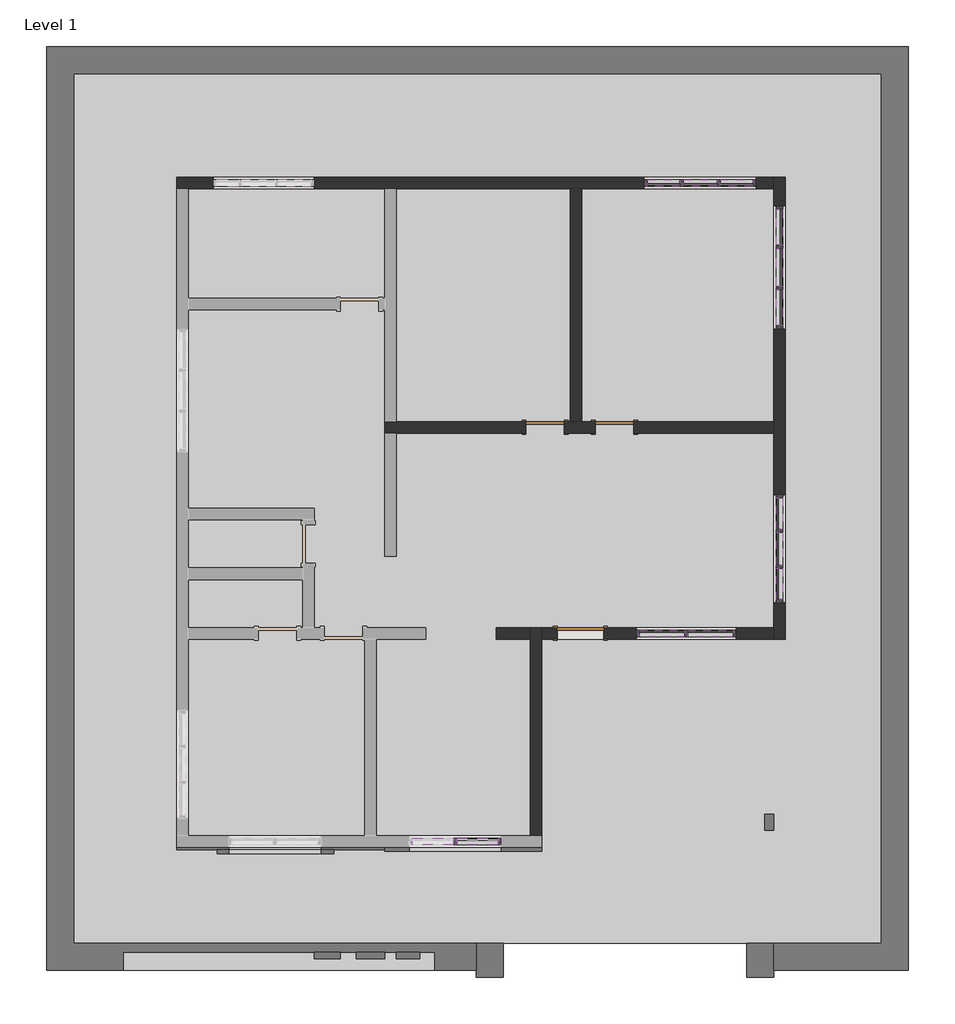
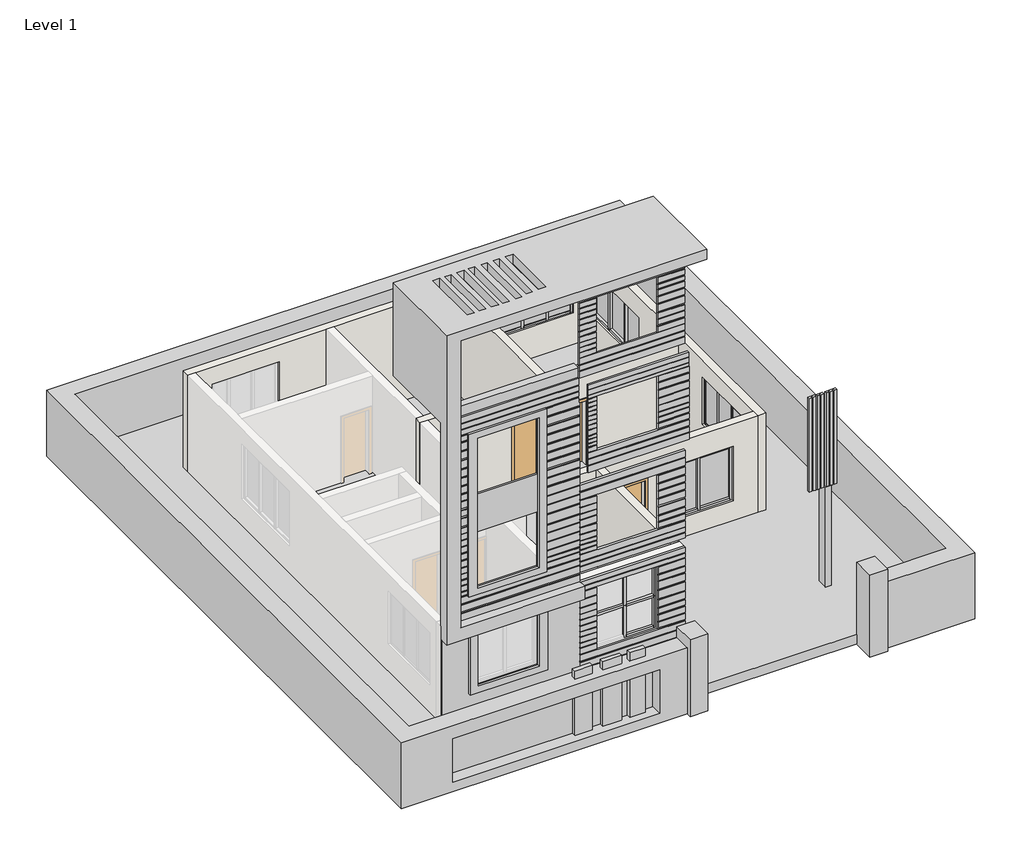
# One storey, part 2 of 2: 46 members, 11 plates, 7 walls, 3 doors, 3 proxies.
"""IFC4 building model written with IfcOpenShell, lengths in millimetres."""

from ifc_helpers import new_model, si_unit, frame, origin, origin_with_axes, place, context, project, spatial, polyline, outline, extrude, faceted_brep, transform, mapped, element, save
from components import generic_models_1_generic_models_1_92ce0f77, generic_models_7_generic_models_7_680a3b92, generic_models_7_generic_models_7_94141b15, generic_models_8_generic_models_8_408287a0, door_a1484949, door_85036156, door_a90ba1ad, member_3f0e0172, member_5215b92c, member_673fd8de, member_e79a7e0a, member_9d02be77, member_7007ad49, member_d44a35f4, member_12fb2005, member_61359a5b, member_26d576e8, member_7f309565, member_d4c304d5, member_f1f71bde, member_07726a47, member_145ad7ec, member_948b814d, member_c17f1be2, member_ad567e07, member_e156fde9, system_panel_glazed_296d4335, system_panel_glazed_a5c0bc7c, system_panel_glazed_82717b58, system_panel_glazed_5516fd1f, system_panel_glazed_95f8db0f, system_panel_glazed_7e52d88a, system_panel_glazed_d1fbebc5

model = new_model("IFC4")

# Units and contexts
model_context = context("Model", 3, world=origin())
ifc_project = project(units=[si_unit("LENGTHUNIT", "METRE", prefix="MILLI")], contexts=[model_context])

# Site, building, storey
site = spatial("IfcSite", under=ifc_project)
building = spatial("IfcBuilding", under=site)
storey = spatial("IfcBuildingStorey", under=building, Name="Level 1", Elevation=0.0)

# Proxies
placement = place(None, origin())
generic_models_1_generic_models_1_shape = generic_models_1_generic_models_1_92ce0f77(model_context)
element("IfcBuildingElementProxy", 1, Name="Generic Models 1 : Generic Models 1", ObjectType="Generic Models 1 : Generic Models 1", at=placement, inside=storey, context=model_context, shape_type="MappedRepresentation", body=[
    mapped(generic_models_1_generic_models_1_shape, transform((0.0, 0.0, 0.0), x_axis=(1.0, 0.0, 0.0), y_axis=(0.0, 1.0, 0.0), z_axis=(0.0, 0.0, 1.0))),
])
generic_models_7_generic_models_7_shape = generic_models_7_generic_models_7_680a3b92(model_context)
generic_models_7_generic_models_7_2_shape = generic_models_7_generic_models_7_94141b15(model_context)
element("IfcBuildingElementProxy", 2, Name="Generic Models 7 : Generic Models 7", ObjectType="Generic Models 7 : Generic Models 7", at=placement, inside=storey, context=model_context, shape_type="MappedRepresentation", body=[
    mapped(generic_models_7_generic_models_7_shape, transform((0.0, 0.0, 0.0), x_axis=(1.0, 0.0, 0.0), y_axis=(0.0, 1.0, 0.0), z_axis=(0.0, 0.0, 1.0))),
    mapped(generic_models_7_generic_models_7_2_shape, transform((0.0, 0.0, 0.0), x_axis=(1.0, 0.0, 0.0), y_axis=(0.0, 1.0, 0.0), z_axis=(0.0, 0.0, 1.0))),
])
generic_models_8_generic_models_8_shape = generic_models_8_generic_models_8_408287a0(model_context)
element("IfcBuildingElementProxy", 3, Name="Generic Models 8 : Generic Models 8", ObjectType="Generic Models 8 : Generic Models 8", at=placement, inside=storey, context=model_context, shape_type="MappedRepresentation", body=[
    mapped(generic_models_8_generic_models_8_shape, transform((0.0, 0.0, 0.0), x_axis=(1.0, 0.0, 0.0), y_axis=(0.0, 1.0, 0.0), z_axis=(0.0, 0.0, 1.0))),
])

# Doors
door_shape = door_a1484949(model_context)
element("IfcDoor", 4, ObjectType="Single-Flush : 30\" x 80\"", at=placement, inside=storey, context=model_context, shape_type="MappedRepresentation", body=[
    mapped(door_shape, transform((-12995.791855, -5548.3538163, 0.0), x_axis=(1.0, 0.0, 0.0), y_axis=(0.0, 1.0, 0.0), z_axis=(0.0, 0.0, 1.0))),
])
door_2_shape = door_85036156(model_context)
element("IfcDoor", 5, ObjectType="Single-Flush : 30\" x 80\"", at=placement, inside=storey, context=model_context, shape_type="MappedRepresentation", body=[
    mapped(door_2_shape, transform((-11624.191855, -5548.3538163, 0.0), x_axis=(-1.0, 0.0, 0.0), y_axis=(0.0, -1.0, 0.0), z_axis=(0.0, 0.0, 1.0))),
])
door_3_shape = door_a90ba1ad(model_context)
element("IfcDoor", 6, ObjectType="Single-Flush : 36\" x 84\"", at=placement, inside=storey, context=model_context, shape_type="MappedRepresentation", body=[
    mapped(door_3_shape, transform((-12297.291855, -9625.0538163, 50.8), x_axis=(-1.0, 0.0, 0.0), y_axis=(0.0, -1.0, 0.0), z_axis=(0.0, 0.0, 1.0))),
])

# Members
member_shape = member_3f0e0172(model_context)
element("IfcMember", 7, ObjectType="Rectangular Mullion : 2.5\" x 5\" rectangular", at=placement, inside=storey, context=model_context, shape_type="MappedRepresentation", body=[
    mapped(member_shape, transform((-8360.291855, -7561.3038163, 1043.4119261), x_axis=(0.0, 0.0, -1.0), y_axis=(1.0, 0.0, 0.0), z_axis=(0.0, -1.0, 0.0))),
])
element("IfcMember", 8, ObjectType="Rectangular Mullion : 2.5\" x 5\" rectangular", at=placement, inside=storey, context=model_context, shape_type="MappedRepresentation", body=[
    mapped(member_shape, transform((-8360.291855, -8951.9538163, 1043.4119261), x_axis=(0.0, 0.0, -1.0), y_axis=(1.0, 0.0, 0.0), z_axis=(0.0, -1.0, 0.0))),
])
member_2_shape = member_5215b92c(model_context)
element("IfcMember", 9, ObjectType="Rectangular Mullion : 2.5\" x 5\" rectangular", at=placement, inside=storey, context=model_context, shape_type="MappedRepresentation", body=[
    mapped(member_2_shape, transform((-8360.291855, -8272.5038163, 1043.4119261), x_axis=(0.0, 0.0, -1.0), y_axis=(1.0, 0.0, 0.0), z_axis=(0.0, -1.0, 0.0))),
])
member_3_shape = member_673fd8de(model_context)
element("IfcMember", 10, ObjectType="Rectangular Mullion : 2.5\" x 5\" rectangular", at=placement, inside=storey, context=model_context, shape_type="MappedRepresentation", body=[
    mapped(member_3_shape, transform((-8360.291855, -8304.2538163, 1043.4119261), x_axis=(0.0, 1.0, 0.0), y_axis=(1.0, 0.0, 0.0), z_axis=(0.0, 0.0, -1.0))),
])
element("IfcMember", 11, ObjectType="Rectangular Mullion : 2.5\" x 5\" rectangular", at=placement, inside=storey, context=model_context, shape_type="MappedRepresentation", body=[
    mapped(member_3_shape, transform((-8360.291855, -7593.0538163, 1043.4119261), x_axis=(0.0, 1.0, 0.0), y_axis=(1.0, 0.0, 0.0), z_axis=(0.0, 0.0, -1.0))),
])
element("IfcMember", 12, ObjectType="Rectangular Mullion : 2.5\" x 5\" rectangular", at=placement, inside=storey, context=model_context, shape_type="MappedRepresentation", body=[
    mapped(member_2_shape, transform((-8360.291855, -7624.8038163, 2519.2132879), x_axis=(0.0, 0.0, 1.0), y_axis=(1.0, 0.0, 0.0), z_axis=(0.0, 1.0, 0.0))),
])
element("IfcMember", 13, ObjectType="Rectangular Mullion : 2.5\" x 5\" rectangular", at=placement, inside=storey, context=model_context, shape_type="MappedRepresentation", body=[
    mapped(member_shape, transform((-8360.291855, -8336.0038163, 2519.2132879), x_axis=(0.0, 0.0, 1.0), y_axis=(1.0, 0.0, 0.0), z_axis=(0.0, 1.0, 0.0))),
])
element("IfcMember", 14, ObjectType="Rectangular Mullion : 2.5\" x 5\" rectangular", at=placement, inside=storey, context=model_context, shape_type="MappedRepresentation", body=[
    mapped(member_shape, transform((-8360.291855, -6945.3538163, 2519.2132879), x_axis=(0.0, 0.0, 1.0), y_axis=(1.0, 0.0, 0.0), z_axis=(0.0, 1.0, 0.0))),
])
member_4_shape = member_e79a7e0a(model_context)
element("IfcMember", 15, ObjectType="Rectangular Mullion : 2.5\" x 5\" rectangular", at=placement, inside=storey, context=model_context, shape_type="MappedRepresentation", body=[
    mapped(member_4_shape, transform((-8360.291855, -6881.8538163, 1043.4119261), x_axis=(0.0, 1.0, 0.0), y_axis=(1.0, 0.0, 0.0), z_axis=(0.0, 0.0, -1.0))),
])
element("IfcMember", 16, ObjectType="Rectangular Mullion : 2.5\" x 5\" rectangular", at=placement, inside=storey, context=model_context, shape_type="MappedRepresentation", body=[
    mapped(member_4_shape, transform((-8360.291855, -9015.4538163, 2519.2132879), x_axis=(0.0, -1.0, 0.0), y_axis=(1.0, 0.0, 0.0), z_axis=(0.0, 0.0, 1.0))),
])
member_5_shape = member_9d02be77(model_context)
element("IfcMember", 17, ObjectType="Rectangular Mullion : 2.5\" x 5\" rectangular", at=placement, inside=storey, context=model_context, shape_type="MappedRepresentation", body=[
    mapped(member_5_shape, transform((-8360.291855, -2011.4038163, 996.5765581), x_axis=(0.0, 0.0, -1.0), y_axis=(-1.0, 0.0, 0.0), z_axis=(0.0, 1.0, 0.0))),
])
member_6_shape = member_7007ad49(model_context)
element("IfcMember", 18, ObjectType="Rectangular Mullion : 2.5\" x 5\" rectangular", at=placement, inside=storey, context=model_context, shape_type="MappedRepresentation", body=[
    mapped(member_6_shape, transform((-8360.291855, -2824.2038163, 996.5765581), x_axis=(0.0, 0.0, -1.0), y_axis=(-1.0, 0.0, 0.0), z_axis=(0.0, 1.0, 0.0))),
])
element("IfcMember", 19, ObjectType="Rectangular Mullion : 2.5\" x 5\" rectangular", at=placement, inside=storey, context=model_context, shape_type="MappedRepresentation", body=[
    mapped(member_6_shape, transform((-8360.291855, -1230.3538163, 996.5765581), x_axis=(0.0, 0.0, -1.0), y_axis=(-1.0, 0.0, 0.0), z_axis=(0.0, 1.0, 0.0))),
])
member_7_shape = member_d44a35f4(model_context)
element("IfcMember", 20, ObjectType="Rectangular Mullion : 2.5\" x 5\" rectangular", at=placement, inside=storey, context=model_context, shape_type="MappedRepresentation", body=[
    mapped(member_7_shape, transform((-8360.291855, -1979.6538163, 996.5765581), x_axis=(0.0, -1.0, 0.0), y_axis=(-1.0, 0.0, 0.0), z_axis=(0.0, 0.0, -1.0))),
])
element("IfcMember", 21, ObjectType="Rectangular Mullion : 2.5\" x 5\" rectangular", at=placement, inside=storey, context=model_context, shape_type="MappedRepresentation", body=[
    mapped(member_7_shape, transform((-8360.291855, -2792.4538163, 996.5765581), x_axis=(0.0, -1.0, 0.0), y_axis=(-1.0, 0.0, 0.0), z_axis=(0.0, 0.0, -1.0))),
])
element("IfcMember", 22, ObjectType="Rectangular Mullion : 2.5\" x 5\" rectangular", at=placement, inside=storey, context=model_context, shape_type="MappedRepresentation", body=[
    mapped(member_6_shape, transform((-8360.291855, -1947.9038163, 2408.3673873), x_axis=(0.0, 0.0, 1.0), y_axis=(-1.0, 0.0, 0.0), z_axis=(0.0, -1.0, 0.0))),
])
element("IfcMember", 23, ObjectType="Rectangular Mullion : 2.5\" x 5\" rectangular", at=placement, inside=storey, context=model_context, shape_type="MappedRepresentation", body=[
    mapped(member_6_shape, transform((-8360.291855, -3541.7538163, 2408.3673873), x_axis=(0.0, 0.0, 1.0), y_axis=(-1.0, 0.0, 0.0), z_axis=(0.0, -1.0, 0.0))),
])
element("IfcMember", 24, ObjectType="Rectangular Mullion : 2.5\" x 5\" rectangular", at=placement, inside=storey, context=model_context, shape_type="MappedRepresentation", body=[
    mapped(member_5_shape, transform((-8360.291855, -2760.7038163, 2408.3673873), x_axis=(0.0, 0.0, 1.0), y_axis=(-1.0, 0.0, 0.0), z_axis=(0.0, -1.0, 0.0))),
])
member_8_shape = member_12fb2005(model_context)
element("IfcMember", 25, ObjectType="Rectangular Mullion : 2.5\" x 5\" rectangular", at=placement, inside=storey, context=model_context, shape_type="MappedRepresentation", body=[
    mapped(member_8_shape, transform((-8360.291855, -3605.2538163, 996.5765581), x_axis=(0.0, -1.0, 0.0), y_axis=(-1.0, 0.0, 0.0), z_axis=(0.0, 0.0, -1.0))),
])
element("IfcMember", 26, ObjectType="Rectangular Mullion : 2.5\" x 5\" rectangular", at=placement, inside=storey, context=model_context, shape_type="MappedRepresentation", body=[
    mapped(member_8_shape, transform((-8360.291855, -1166.8538163, 2408.3673873), x_axis=(0.0, 1.0, 0.0), y_axis=(-1.0, 0.0, 0.0), z_axis=(0.0, 0.0, 1.0))),
])
member_9_shape = member_61359a5b(model_context)
element("IfcMember", 27, ObjectType="Rectangular Mullion : 2.5\" x 5\" rectangular", at=placement, inside=storey, context=model_context, shape_type="MappedRepresentation", body=[
    mapped(member_9_shape, transform((-9526.5751883, -709.6538163, 2499.4975793), x_axis=(0.0, 0.0, 1.0), y_axis=(0.0, 1.0, 0.0), z_axis=(-1.0, 0.0, 0.0))),
])
element("IfcMember", 28, ObjectType="Rectangular Mullion : 2.5\" x 5\" rectangular", at=placement, inside=storey, context=model_context, shape_type="MappedRepresentation", body=[
    mapped(member_9_shape, transform((-10976.491855, -709.6538163, 2499.4975793), x_axis=(0.0, 0.0, 1.0), y_axis=(0.0, 1.0, 0.0), z_axis=(-1.0, 0.0, 0.0))),
])
member_10_shape = member_26d576e8(model_context)
element("IfcMember", 29, ObjectType="Rectangular Mullion : 2.5\" x 5\" rectangular", at=placement, inside=storey, context=model_context, shape_type="MappedRepresentation", body=[
    mapped(member_10_shape, transform((-10267.4085217, -709.6538163, 2499.4975793), x_axis=(0.0, 0.0, 1.0), y_axis=(0.0, 1.0, 0.0), z_axis=(-1.0, 0.0, 0.0))),
])
member_11_shape = member_7f309565(model_context)
element("IfcMember", 30, ObjectType="Rectangular Mullion : 2.5\" x 5\" rectangular", at=placement, inside=storey, context=model_context, shape_type="MappedRepresentation", body=[
    mapped(member_11_shape, transform((-10299.1585217, -709.6538163, 985.9213876), x_axis=(-1.0, 0.0, 0.0), y_axis=(0.0, 1.0, 0.0), z_axis=(0.0, 0.0, -1.0))),
])
element("IfcMember", 31, ObjectType="Rectangular Mullion : 2.5\" x 5\" rectangular", at=placement, inside=storey, context=model_context, shape_type="MappedRepresentation", body=[
    mapped(member_11_shape, transform((-9558.3251883, -709.6538163, 985.9213876), x_axis=(-1.0, 0.0, 0.0), y_axis=(0.0, 1.0, 0.0), z_axis=(0.0, 0.0, -1.0))),
])
element("IfcMember", 32, ObjectType="Rectangular Mullion : 2.5\" x 5\" rectangular", at=placement, inside=storey, context=model_context, shape_type="MappedRepresentation", body=[
    mapped(member_10_shape, transform((-9590.0751883, -709.6538163, 985.9213876), x_axis=(0.0, 0.0, -1.0), y_axis=(0.0, 1.0, 0.0), z_axis=(1.0, 0.0, 0.0))),
])
element("IfcMember", 33, ObjectType="Rectangular Mullion : 2.5\" x 5\" rectangular", at=placement, inside=storey, context=model_context, shape_type="MappedRepresentation", body=[
    mapped(member_9_shape, transform((-10330.9085217, -709.6538163, 985.9213876), x_axis=(0.0, 0.0, -1.0), y_axis=(0.0, 1.0, 0.0), z_axis=(1.0, 0.0, 0.0))),
])
element("IfcMember", 34, ObjectType="Rectangular Mullion : 2.5\" x 5\" rectangular", at=placement, inside=storey, context=model_context, shape_type="MappedRepresentation", body=[
    mapped(member_9_shape, transform((-8880.991855, -709.6538163, 985.9213876), x_axis=(0.0, 0.0, -1.0), y_axis=(0.0, 1.0, 0.0), z_axis=(1.0, 0.0, 0.0))),
])
member_12_shape = member_d4c304d5(model_context)
element("IfcMember", 35, ObjectType="Rectangular Mullion : 2.5\" x 5\" rectangular", at=placement, inside=storey, context=model_context, shape_type="MappedRepresentation", body=[
    mapped(member_12_shape, transform((-11039.991855, -709.6538163, 985.9213876), x_axis=(-1.0, 0.0, 0.0), y_axis=(0.0, 1.0, 0.0), z_axis=(0.0, 0.0, -1.0))),
])
element("IfcMember", 36, ObjectType="Rectangular Mullion : 2.5\" x 5\" rectangular", at=placement, inside=storey, context=model_context, shape_type="MappedRepresentation", body=[
    mapped(member_12_shape, transform((-8817.491855, -709.6538163, 2499.4975793), x_axis=(1.0, 0.0, 0.0), y_axis=(0.0, 1.0, 0.0), z_axis=(0.0, 0.0, 1.0))),
])
member_13_shape = member_f1f71bde(model_context)
element("IfcMember", 37, ObjectType="Rectangular Mullion : 2.5\" x 5\" rectangular", at=placement, inside=storey, context=model_context, shape_type="MappedRepresentation", body=[
    mapped(member_13_shape, transform((-10233.541855, -9625.0538163, 2332.3247485), x_axis=(0.0, 0.0, 1.0), y_axis=(0.0, -1.0, 0.0), z_axis=(1.0, 0.0, 0.0))),
])
element("IfcMember", 38, ObjectType="Rectangular Mullion : 2.5\" x 5\" rectangular", at=placement, inside=storey, context=model_context, shape_type="MappedRepresentation", body=[
    mapped(member_13_shape, transform((-9274.691855, -9625.0538163, 2332.3247485), x_axis=(0.0, 0.0, 1.0), y_axis=(0.0, -1.0, 0.0), z_axis=(1.0, 0.0, 0.0))),
])
member_14_shape = member_07726a47(model_context)
element("IfcMember", 39, ObjectType="Rectangular Mullion : 2.5\" x 5\" rectangular", at=placement, inside=storey, context=model_context, shape_type="MappedRepresentation", body=[
    mapped(member_14_shape, transform((-10201.791855, -9625.0538163, 631.9229902), x_axis=(1.0, 0.0, 0.0), y_axis=(0.0, -1.0, 0.0), z_axis=(0.0, 0.0, -1.0))),
])
element("IfcMember", 40, ObjectType="Rectangular Mullion : 2.5\" x 5\" rectangular", at=placement, inside=storey, context=model_context, shape_type="MappedRepresentation", body=[
    mapped(member_13_shape, transform((-10170.041855, -9625.0538163, 631.9229902), x_axis=(0.0, 0.0, -1.0), y_axis=(0.0, -1.0, 0.0), z_axis=(-1.0, 0.0, 0.0))),
])
element("IfcMember", 41, ObjectType="Rectangular Mullion : 2.5\" x 5\" rectangular", at=placement, inside=storey, context=model_context, shape_type="MappedRepresentation", body=[
    mapped(member_13_shape, transform((-11128.891855, -9625.0538163, 631.9229902), x_axis=(0.0, 0.0, -1.0), y_axis=(0.0, -1.0, 0.0), z_axis=(-1.0, 0.0, 0.0))),
])
member_15_shape = member_145ad7ec(model_context)
element("IfcMember", 42, ObjectType="Rectangular Mullion : 2.5\" x 5\" rectangular", at=placement, inside=storey, context=model_context, shape_type="MappedRepresentation", body=[
    mapped(member_15_shape, transform((-9211.191855, -9625.0538163, 631.9229902), x_axis=(1.0, 0.0, 0.0), y_axis=(0.0, -1.0, 0.0), z_axis=(0.0, 0.0, -1.0))),
])
element("IfcMember", 43, ObjectType="Rectangular Mullion : 2.5\" x 5\" rectangular", at=placement, inside=storey, context=model_context, shape_type="MappedRepresentation", body=[
    mapped(member_15_shape, transform((-11192.391855, -9625.0538163, 2332.3247485), x_axis=(-1.0, 0.0, 0.0), y_axis=(0.0, -1.0, 0.0), z_axis=(0.0, 0.0, 1.0))),
])
member_16_shape = member_948b814d(model_context)
element("IfcMember", 44, ObjectType="Rectangular Mullion : 2.5\" x 5\" rectangular", at=placement, inside=storey, context=model_context, shape_type="MappedRepresentation", body=[
    mapped(member_16_shape, transform((-14773.791855, -13739.8538163, 1742.3683755), x_axis=(1.0, 0.0, 0.0), y_axis=(0.0, -1.0, 0.0), z_axis=(0.0, 0.0, -1.0))),
])
member_17_shape = member_c17f1be2(model_context)
element("IfcMember", 45, ObjectType="Rectangular Mullion : 2.5\" x 5\" rectangular", at=placement, inside=storey, context=model_context, shape_type="MappedRepresentation", body=[
    mapped(member_17_shape, transform((-14805.541855, -13739.8538163, 2743.3706019), x_axis=(0.0, 0.0, 1.0), y_axis=(0.0, -1.0, 0.0), z_axis=(1.0, 0.0, 0.0))),
])
element("IfcMember", 46, ObjectType="Rectangular Mullion : 2.5\" x 5\" rectangular", at=placement, inside=storey, context=model_context, shape_type="MappedRepresentation", body=[
    mapped(member_17_shape, transform((-13922.891855, -13739.8538163, 2743.3706019), x_axis=(0.0, 0.0, 1.0), y_axis=(0.0, -1.0, 0.0), z_axis=(1.0, 0.0, 0.0))),
])
member_18_shape = member_ad567e07(model_context)
element("IfcMember", 47, ObjectType="Rectangular Mullion : 2.5\" x 5\" rectangular", at=placement, inside=storey, context=model_context, shape_type="MappedRepresentation", body=[
    mapped(member_18_shape, transform((-13922.891855, -13739.8538163, 1742.3683755), x_axis=(0.0, 0.0, 1.0), y_axis=(0.0, -1.0, 0.0), z_axis=(1.0, 0.0, 0.0))),
])
element("IfcMember", 48, ObjectType="Rectangular Mullion : 2.5\" x 5\" rectangular", at=placement, inside=storey, context=model_context, shape_type="MappedRepresentation", body=[
    mapped(member_18_shape, transform((-14805.541855, -13739.8538163, 1742.3683755), x_axis=(0.0, 0.0, 1.0), y_axis=(0.0, -1.0, 0.0), z_axis=(1.0, 0.0, 0.0))),
])
member_19_shape = member_e156fde9(model_context)
element("IfcMember", 49, ObjectType="Rectangular Mullion : 2.5\" x 5\" rectangular", at=placement, inside=storey, context=model_context, shape_type="MappedRepresentation", body=[
    mapped(member_19_shape, transform((-13859.391855, -13739.8538163, 1742.3683755), x_axis=(1.0, 0.0, 0.0), y_axis=(0.0, -1.0, 0.0), z_axis=(0.0, 0.0, -1.0))),
])
element("IfcMember", 50, ObjectType="Rectangular Mullion : 2.5\" x 5\" rectangular", at=placement, inside=storey, context=model_context, shape_type="MappedRepresentation", body=[
    mapped(member_16_shape, transform((-14773.791855, -13739.8538163, 741.3661492), x_axis=(1.0, 0.0, 0.0), y_axis=(0.0, -1.0, 0.0), z_axis=(0.0, 0.0, -1.0))),
])
element("IfcMember", 51, ObjectType="Rectangular Mullion : 2.5\" x 5\" rectangular", at=placement, inside=storey, context=model_context, shape_type="MappedRepresentation", body=[
    mapped(member_17_shape, transform((-14742.041855, -13739.8538163, 741.3661492), x_axis=(0.0, 0.0, -1.0), y_axis=(0.0, -1.0, 0.0), z_axis=(-1.0, 0.0, 0.0))),
])
element("IfcMember", 52, ObjectType="Rectangular Mullion : 2.5\" x 5\" rectangular", at=placement, inside=storey, context=model_context, shape_type="MappedRepresentation", body=[
    mapped(member_19_shape, transform((-13859.391855, -13739.8538163, 741.3661492), x_axis=(1.0, 0.0, 0.0), y_axis=(0.0, -1.0, 0.0), z_axis=(0.0, 0.0, -1.0))),
])

# Plates
system_panel_glazed_shape = system_panel_glazed_296d4335(model_context)
element("IfcPlate", 53, ObjectType="System Panel : Glazed", at=placement, inside=storey, context=model_context, shape_type="MappedRepresentation", body=[
    mapped(system_panel_glazed_shape, transform((-8360.291855, -8643.9788163, 1106.9119261), x_axis=(0.0, 1.0, 0.0), y_axis=(-1.0, 0.0, 0.0), z_axis=(0.0, 0.0, 1.0))),
])
element("IfcPlate", 54, ObjectType="System Panel : Glazed", at=placement, inside=storey, context=model_context, shape_type="MappedRepresentation", body=[
    mapped(system_panel_glazed_shape, transform((-8360.291855, -7253.3288163, 1106.9119261), x_axis=(0.0, 1.0, 0.0), y_axis=(-1.0, 0.0, 0.0), z_axis=(0.0, 0.0, 1.0))),
])
system_panel_glazed_2_shape = system_panel_glazed_a5c0bc7c(model_context)
element("IfcPlate", 55, ObjectType="System Panel : Glazed", at=placement, inside=storey, context=model_context, shape_type="MappedRepresentation", body=[
    mapped(system_panel_glazed_2_shape, transform((-8360.291855, -7948.6538163, 1106.9119261), x_axis=(0.0, 1.0, 0.0), y_axis=(-1.0, 0.0, 0.0), z_axis=(0.0, 0.0, 1.0))),
])
system_panel_glazed_3_shape = system_panel_glazed_82717b58(model_context)
element("IfcPlate", 56, ObjectType="System Panel : Glazed", at=placement, inside=storey, context=model_context, shape_type="MappedRepresentation", body=[
    mapped(system_panel_glazed_3_shape, transform((-8360.291855, -1589.1288163, 1060.0765581), x_axis=(0.0, -1.0, 0.0), y_axis=(1.0, 0.0, 0.0), z_axis=(0.0, 0.0, 1.0))),
])
element("IfcPlate", 57, ObjectType="System Panel : Glazed", at=placement, inside=storey, context=model_context, shape_type="MappedRepresentation", body=[
    mapped(system_panel_glazed_3_shape, transform((-8360.291855, -3182.9788163, 1060.0765581), x_axis=(0.0, -1.0, 0.0), y_axis=(1.0, 0.0, 0.0), z_axis=(0.0, 0.0, 1.0))),
])
system_panel_glazed_4_shape = system_panel_glazed_5516fd1f(model_context)
element("IfcPlate", 58, ObjectType="System Panel : Glazed", at=placement, inside=storey, context=model_context, shape_type="MappedRepresentation", body=[
    mapped(system_panel_glazed_4_shape, transform((-8360.291855, -2386.0538163, 1060.0765581), x_axis=(0.0, -1.0, 0.0), y_axis=(1.0, 0.0, 0.0), z_axis=(0.0, 0.0, 1.0))),
])
system_panel_glazed_5_shape = system_panel_glazed_95f8db0f(model_context)
element("IfcPlate", 59, ObjectType="System Panel : Glazed", at=placement, inside=storey, context=model_context, shape_type="MappedRepresentation", body=[
    mapped(system_panel_glazed_5_shape, transform((-9203.7835217, -709.6538163, 1049.4213876), x_axis=(-1.0, 0.0, 0.0), y_axis=(0.0, -1.0, 0.0), z_axis=(0.0, 0.0, 1.0))),
])
element("IfcPlate", 60, ObjectType="System Panel : Glazed", at=placement, inside=storey, context=model_context, shape_type="MappedRepresentation", body=[
    mapped(system_panel_glazed_5_shape, transform((-10653.7001883, -709.6538163, 1049.4213876), x_axis=(-1.0, 0.0, 0.0), y_axis=(0.0, -1.0, 0.0), z_axis=(0.0, 0.0, 1.0))),
])
system_panel_glazed_6_shape = system_panel_glazed_7e52d88a(model_context)
element("IfcPlate", 61, ObjectType="System Panel : Glazed", at=placement, inside=storey, context=model_context, shape_type="MappedRepresentation", body=[
    mapped(system_panel_glazed_6_shape, transform((-9928.741855, -709.6538163, 1049.4213876), x_axis=(-1.0, 0.0, 0.0), y_axis=(0.0, -1.0, 0.0), z_axis=(0.0, 0.0, 1.0))),
])
system_panel_glazed_7_shape = system_panel_glazed_d1fbebc5(model_context)
element("IfcPlate", 62, ObjectType="System Panel : Glazed", at=placement, inside=storey, context=model_context, shape_type="MappedRepresentation", body=[
    mapped(system_panel_glazed_7_shape, transform((-10681.216855, -9625.0538163, 695.4229902), x_axis=(1.0, 0.0, 0.0), y_axis=(0.0, 1.0, 0.0), z_axis=(0.0, 0.0, 1.0))),
])
element("IfcPlate", 63, ObjectType="System Panel : Glazed", at=placement, inside=storey, context=model_context, shape_type="MappedRepresentation", body=[
    mapped(system_panel_glazed_7_shape, transform((-9722.366855, -9625.0538163, 695.4229902), x_axis=(1.0, 0.0, 0.0), y_axis=(0.0, 1.0, 0.0), z_axis=(0.0, 0.0, 1.0))),
])

# Walls
element("IfcWall", 64, ObjectType="9\"", at=placement, inside=storey, context=model_context, shape_type="Brep", body=[
    faceted_brep([(-8474.591855, -595.3538163, 0.0), (-20285.591855, -595.3538163, 0.0), (-20285.591855, -595.3538163, 3048.0), (-8474.591855, -595.3538163, 3048.0), (-8817.491855, -595.3538163, 985.9213876), (-8817.491855, -595.3538163, 2499.4975793), (-11039.991855, -595.3538163, 2499.4975793), (-11039.991855, -595.3538163, 985.9213876), (-19561.691855, -595.3538163, 2512.1183195), (-19561.691855, -595.3538163, 954.7607085), (-17567.791855, -595.3538163, 954.7607085), (-17567.791855, -595.3538163, 2512.1183195), (-20285.591855, -823.9538163, 0.0), (-20056.991855, -823.9538163, 0.0), (-16170.791855, -823.9538163, 0.0), (-15942.191855, -823.9538163, 0.0), (-12500.491855, -823.9538163, 0.0), (-12271.891855, -823.9538163, 0.0), (-8474.591855, -823.9538163, 0.0), (-8474.591855, -823.9538163, 3048.0), (-12271.891855, -823.9538163, 3048.0), (-12500.491855, -823.9538163, 3048.0), (-15942.191855, -823.9538163, 3048.0), (-16170.791855, -823.9538163, 3048.0), (-20056.991855, -823.9538163, 3048.0), (-20285.591855, -823.9538163, 3048.0), (-8817.491855, -823.9538163, 2499.4975793), (-8817.491855, -823.9538163, 985.9213876), (-11039.991855, -823.9538163, 985.9213876), (-11039.991855, -823.9538163, 2499.4975793), (-19561.691855, -823.9538163, 954.7607085), (-19561.691855, -823.9538163, 2512.1183195), (-17567.791855, -823.9538163, 2512.1183195), (-17567.791855, -823.9538163, 954.7607085)], [[[0, 1, 2, 3], [4, 5, 6, 7], [8, 9, 10, 11]], [[12, 13, 14, 15, 16, 17, 18, 19, 20, 21, 22, 23, 24, 25], [26, 27, 28, 29], [30, 31, 32, 33]], [[1, 0, 18, 17, 16, 15, 14, 13, 12]], [[3, 2, 25, 24, 23, 22, 21, 20, 19]], [[0, 3, 19, 18]], [[2, 1, 12, 25]], [[4, 27, 26, 5]], [[5, 26, 29, 6]], [[6, 29, 28, 7]], [[27, 4, 7, 28]], [[30, 9, 8, 31]], [[31, 8, 11, 32]], [[10, 33, 32, 11]], [[9, 30, 33, 10]]]),
])
element("IfcWall", 65, ObjectType="9\"", at=placement, inside=storey, context=model_context, shape_type="SweptSolid", body=[
    extrude(outline(polyline([(-13960.991855, -9510.7538163), (-13287.891855, -9510.7538163), (-13287.891855, -9739.3538163), (-13960.991855, -9739.3538163), (-13960.991855, -9510.7538163)])), origin_with_axes(), (0.0, 0.0, 1.0), 3048.0),
])
element("IfcWall", 66, ObjectType="9\"", at=placement, inside=storey, context=model_context, shape_type="Brep", body=[
    faceted_brep([(-13059.291855, -13625.5538163, 0.0), (-13059.291855, -9739.3538163, 0.0), (-13059.291855, -9510.7538163, 0.0), (-13059.291855, -9510.7538163, 3048.0), (-13059.291855, -9739.3538163, 3048.0), (-13059.291855, -13625.5538163, 3048.0), (-13287.891855, -13625.5538163, 0.0), (-13287.891855, -13625.5538163, 3048.0), (-13287.891855, -9739.3538163, 3048.0), (-13287.891855, -9510.7538163, 3048.0), (-13287.891855, -9510.7538163, 0.0), (-13287.891855, -9739.3538163, 0.0)], [[[0, 1, 2, 3, 4, 5]], [[6, 7, 8, 9, 10, 11]], [[2, 1, 0, 6, 11, 10]], [[5, 4, 3, 9, 8, 7]], [[0, 5, 7, 6]], [[3, 2, 10, 9]]]),
])
element("IfcWall", 67, ObjectType="9\"", at=placement, inside=storey, context=model_context, shape_type="SweptSolid", body=[
    extrude(outline(polyline([(0.0, -13059.291855), (0.0, -8474.591855), (3048.0, -8474.591855), (3048.0, -13059.291855), (0.0, -13059.291855)]), holes=[polyline([(50.8, -11840.091855), (50.8, -12754.491855), (2184.4, -12754.491855), (2184.4, -11840.091855), (50.8, -11840.091855)]), polyline([(631.9229902, -11192.391855), (2332.3247485, -11192.391855), (2332.3247485, -9211.191855), (631.9229902, -9211.191855), (631.9229902, -11192.391855)])]), frame((0.0, -9739.3538163, 0.0), z_axis=(0.0, 1.0, 0.0), x_axis=(0.0, 0.0, 1.0)), (0.0, 0.0, 1.0), 228.6),
])
element("IfcWall", 68, ObjectType="9\"", at=placement, inside=storey, context=model_context, shape_type="Brep", body=[
    faceted_brep([(-12005.191855, -5434.0538163, 2032.0), (-12005.191855, -5434.0538163, 0.0), (-12271.891855, -5434.0538163, 0.0), (-12500.491855, -5434.0538163, 0.0), (-12614.791855, -5434.0538163, 0.0), (-12614.791855, -5434.0538163, 2032.0), (-13376.791855, -5434.0538163, 2032.0), (-13376.791855, -5434.0538163, 0.0), (-15942.191855, -5434.0538163, 0.0), (-16170.791855, -5434.0538163, 0.0), (-16170.791855, -5434.0538163, 3048.0), (-15942.191855, -5434.0538163, 3048.0), (-12500.491855, -5434.0538163, 3048.0), (-12271.891855, -5434.0538163, 3048.0), (-8474.591855, -5434.0538163, 3048.0), (-8474.591855, -5434.0538163, 0.0), (-11243.191855, -5434.0538163, 0.0), (-11243.191855, -5434.0538163, 2032.0), (-12614.791855, -5662.6538163, 0.0), (-12005.191855, -5662.6538163, 0.0), (-12005.191855, -5662.6538163, 2032.0), (-11243.191855, -5662.6538163, 2032.0), (-11243.191855, -5662.6538163, 0.0), (-8474.591855, -5662.6538163, 0.0), (-8474.591855, -5662.6538163, 3048.0), (-15942.191855, -5662.6538163, 3048.0), (-16170.791855, -5662.6538163, 3048.0), (-16170.791855, -5662.6538163, 0.0), (-15942.191855, -5662.6538163, 0.0), (-13376.791855, -5662.6538163, 0.0), (-13376.791855, -5662.6538163, 2032.0), (-12614.791855, -5662.6538163, 2032.0)], [[[0, 1, 2, 3, 4, 5, 6, 7, 8, 9, 10, 11, 12, 13, 14, 15, 16, 17]], [[18, 19, 20, 21, 22, 23, 24, 25, 26, 27, 28, 29, 30, 31]], [[29, 28, 27, 9, 8, 7]], [[16, 15, 23, 22]], [[4, 3, 2, 1, 19, 18]], [[14, 13, 12, 11, 10, 26, 25, 24]], [[15, 14, 24, 23]], [[10, 9, 27, 26]], [[5, 4, 18, 31]], [[6, 5, 31, 30]], [[7, 6, 30, 29]], [[20, 19, 1, 0]], [[21, 20, 0, 17]], [[22, 21, 17, 16]]]),
])
element("IfcWall", 69, ObjectType="9\"", at=placement, inside=storey, context=model_context, shape_type="SweptSolid", body=[
    extrude(outline(polyline([(-12500.491855, -5434.0538163), (-12500.491855, -823.9538163), (-12271.891855, -823.9538163), (-12271.891855, -5434.0538163), (-12500.491855, -5434.0538163)])), origin_with_axes(), (0.0, 0.0, 1.0), 3048.0),
])
element("IfcWall", 70, ObjectType="9\"", at=placement, inside=storey, context=model_context, shape_type="Brep", body=[
    faceted_brep([(-8245.991855, -9739.3538163, 0.0), (-8245.991855, -595.3538163, 0.0), (-8245.991855, -595.3538163, 3048.0), (-8245.991855, -9739.3538163, 3048.0), (-8245.991855, -9015.4538163, 1043.4119261), (-8245.991855, -9015.4538163, 2519.2132879), (-8245.991855, -6881.8538163, 2519.2132879), (-8245.991855, -6881.8538163, 1043.4119261), (-8245.991855, -1166.8538163, 2408.3673873), (-8245.991855, -1166.8538163, 996.5765581), (-8245.991855, -3605.2538163, 996.5765581), (-8245.991855, -3605.2538163, 2408.3673873), (-8474.591855, -595.3538163, 0.0), (-8474.591855, -823.9538163, 0.0), (-8474.591855, -5434.0538163, 0.0), (-8474.591855, -5662.6538163, 0.0), (-8474.591855, -9510.7538163, 0.0), (-8474.591855, -9739.3538163, 0.0), (-8474.591855, -9739.3538163, 3048.0), (-8474.591855, -9510.7538163, 3048.0), (-8474.591855, -5662.6538163, 3048.0), (-8474.591855, -5434.0538163, 3048.0), (-8474.591855, -823.9538163, 3048.0), (-8474.591855, -595.3538163, 3048.0), (-8474.591855, -9015.4538163, 2519.2132879), (-8474.591855, -9015.4538163, 1043.4119261), (-8474.591855, -6881.8538163, 1043.4119261), (-8474.591855, -6881.8538163, 2519.2132879), (-8474.591855, -1166.8538163, 996.5765581), (-8474.591855, -1166.8538163, 2408.3673873), (-8474.591855, -3605.2538163, 2408.3673873), (-8474.591855, -3605.2538163, 996.5765581)], [[[0, 1, 2, 3], [4, 5, 6, 7], [8, 9, 10, 11]], [[12, 13, 14, 15, 16, 17, 18, 19, 20, 21, 22, 23], [24, 25, 26, 27], [28, 29, 30, 31]], [[1, 0, 17, 16, 15, 14, 13, 12]], [[3, 2, 23, 22, 21, 20, 19, 18]], [[0, 3, 18, 17]], [[2, 1, 12, 23]], [[4, 25, 24, 5]], [[5, 24, 27, 6]], [[6, 27, 26, 7]], [[25, 4, 7, 26]], [[28, 9, 8, 29]], [[29, 8, 11, 30]], [[30, 11, 10, 31]], [[9, 28, 31, 10]]]),
])

save(model, "model.ifc")

# Revit data of these elements
# Type "Single-Flush : 30\" x 80\""
#   Type Mark = "5"
#   Construction Type Id = "MDOOR"
#   Assembly Code = "C1020"
#   Analytic Construction = "Metal"
#   Thickness = 0' - 2"
#   Heat Transfer Coefficient (U) = 0.651978 BTU/(h·ft²·°F)
#   Height = 6' - 8"
#   Trim Projection Ext = 0' - 1"
#   Trim Projection Int = 0' - 1"
#   Trim Width = 0' - 3"
#   Width = 2' - 6"
#   Define Thermal Properties by = 1
#   Define Thermal Properties by = 1
#   Door Material = Door - Panel
#   Frame Material = Door - Frame
#   Visual Light Transmittance = 0
#   Solar Heat Gain Coefficient = 0
#   Function = (empty or 0)
#   Wall Closure = (empty or 0)
# Type "Single-Flush : 36\" x 84\""
#   Type Mark = "1"
#   Construction Type Id = "MDOOR"
#   Assembly Code = "C1020"
#   Analytic Construction = "Metal"
#   Thickness = 0' - 2"
#   Heat Transfer Coefficient (U) = 0.651978 BTU/(h·ft²·°F)
#   Height = 7' - 0"
#   Trim Projection Ext = 0' - 1"
#   Trim Projection Int = 0' - 1"
#   Trim Width = 0' - 3"
#   Width = 3' - 0"
#   Define Thermal Properties by = 1
#   Define Thermal Properties by = 1
#   Door Material = Door - Panel
#   Frame Material = Door - Frame
#   Visual Light Transmittance = 0
#   Solar Heat Gain Coefficient = 0
#   Function = (empty or 0)
#   Wall Closure = (empty or 0)
# Type "Rectangular Mullion : 2.5\" x 5\" rectangular"
#   built-in parameter 1007304 = 0.416667 (stored number, unit not read)
#   built-in parameter 1007301 = 0.104167 (stored number, unit not read)
#   built-in parameter 1007300 = 0.104167 (stored number, unit not read)
# Type "System Panel : Glazed"
#   Construction Type Id = "GSP4R"
#   Analytic Construction = "1/8 in Pilkington single glazing"
#   Visual Light Transmittance = 0.9
#   Solar Heat Gain Coefficient = 0.86
#   Heat Transfer Coefficient (U) = 1.18115 BTU/(h·ft²·°F)
#   Define Thermal Properties by = 1
# Type "9\""
#   Assembly Code = "B2010"
#   Layers, outside or top first: 0' - 9" no material (function 1)
# Element 1 (IfcBuildingElementProxy, "Generic Models 1 : Generic Models 1")
#   Phase Created = New Construction
# Element 2 (IfcBuildingElementProxy, "Generic Models 7 : Generic Models 7")
#   Phase Created = New Construction
# Element 3 (IfcBuildingElementProxy, "Generic Models 8 : Generic Models 8")
#   Phase Created = New Construction
# Elements 4, 5 (IfcDoor, "Single-Flush : 30\" x 80\"")
#   Phase Created = New Construction
#   Materials on its faces: "Door - Frame", "Door - Panel"
# Element 6 (IfcDoor, "Single-Flush : 36\" x 84\"")
#   Phase Created = New Construction
#   Materials on its faces: "Door - Frame", "Door - Panel"
# Elements 7, 8, 9, 10, 11, 12, 13, 14, 15, 16, 17, 18, 19, 20, 21, 22, 23, 24, 25, 26, 27, 28, 29, 30, 31, 32, 33, 34, 35, 36, 37, 38, 39, 40, 41, 42, 43, 44, 45, 46, 47, 48, 49, 50, 51, 52 (IfcMember, "Rectangular Mullion : 2.5\" x 5\" rectangular")
#   Phase Created = New Construction
#   Materials on its faces: "Aluminum"
# Elements 53, 54, 55, 56, 57, 58, 59, 60, 61, 62, 63 (IfcPlate, "System Panel : Glazed")
#   Phase Created = New Construction
#   Materials on its faces: "Glass"
# Elements 64, 65, 66, 67, 68, 69, 70 (IfcWall, "9\"")
#   Top Offset = 0' - 0"
#   Base Offset = 0' - 0"
#   Unconnected Height = 10' - 0"
#   wall height = 10' - 0"
#   Phase Created = New Construction
#   Base Constraint = Level 1
#   Materials on its faces: "Default Wall"
# Materials
#   "Door - Panel": class "Wood", colour RGB 210 159 95, transparency 0, Cost = 0
#   "Door - Frame": colour RGB 118 70 51, transparency 0, Cost = 0
#   "Aluminum": class "Metal", colour RGB 247 247 247, transparency 0, Description = "Aluminum 6061", Cost = 0
#   "Glass": class "Glass", colour RGB 0 128 192, transparency 0.75, Description = "Soda Lime Glass", Cost = 0
#   "Default Wall": colour RGB 128 128 128, transparency 0, Cost = 0
